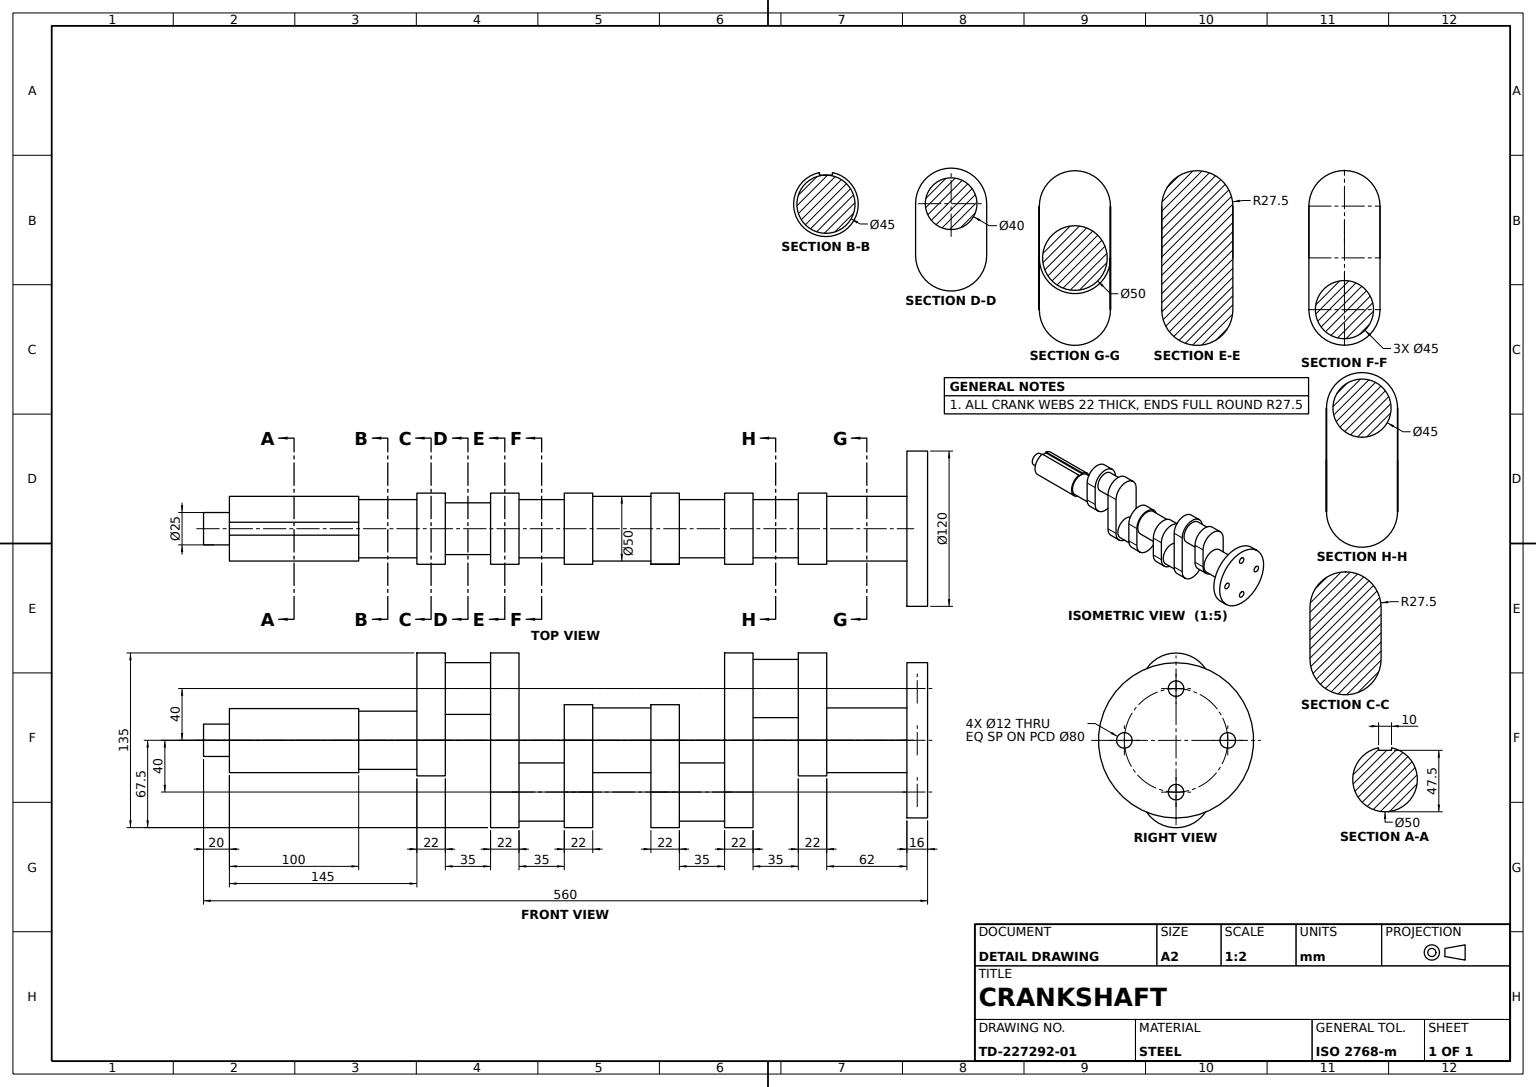
from build123d import *

# Parameters (mm, degrees)
FLANGE_SKETCH_R               = 60
FLANGE_120X16_DEPTH           = 16
FRONT_SHAFT_SKETCH_R          = 25
FRONT_SHAFT_50X62_DEPTH       = 62
CRANK_WEB_1_DEPTH             = 22
CRANKPIN_1_SKETCH_R           = 22.5
CRANKPIN_1_45_DEPTH           = 35
CRANK_WEB_2_DEPTH             = 22
CRANKPIN_2_SKETCH_R           = 22.5
CRANKPIN_2_45_DEPTH           = 35
CRANK_WEB_3_DEPTH             = 22
CENTRE_MAIN_JOURNAL_SKETCH_R  = 25
CENTRE_MAIN_JOURNAL_50_DEPTH  = 45
CRANK_WEB_4_DEPTH             = 22
CRANKPIN_3_SKETCH_R           = 22.5
CRANKPIN_3_45_DEPTH           = 35
CRANK_WEB_5_DEPTH             = 22
CRANKPIN_4_SKETCH_R           = 20
CRANKPIN_4_40_DEPTH           = 35
CRANK_WEB_6_DEPTH             = 22
REAR_SHAFT_SKETCH_R           = 22.5
REAR_SHAFT_45X145_DEPTH       = 145
REAR_START                    = -100
REAR_SHAFT_STEP_SKETCH_R      = 25
REAR_SHAFT_STEP_50X100_DEPTH  = 100
REAR_SHAFT_PROFILE_CUT_DEPTH  = 100
END_STUB_SKETCH_R             = 12.5
END_STUB_25X20_DEPTH          = 20
FLANGE_BOLT_HOLES_SKETCH_R    = 6
FLANGE_BOLT_HOLES_4X_12_DEPTH = 20


with BuildPart() as part:
    # Flange Sketch → Flange Ø120x16 (new body)
    with BuildSketch(Plane.XY):
        Circle(FLANGE_SKETCH_R)
    extrude(amount=FLANGE_120X16_DEPTH)

    # Front Shaft Sketch → Front Shaft Ø50x62 (add)
    with BuildSketch(Plane.XY.offset(16)):
        Circle(FRONT_SHAFT_SKETCH_R)
    extrude(amount=FRONT_SHAFT_50X62_DEPTH)

    # Crank Web 1 Sketch → Crank Web 1 (add)
    with BuildSketch(Plane.XY.offset(78)):
        with BuildLine():
            Line((0, -27.5), (-40, -27.5))
            ThreePointArc((-40, -27.5), (-67.5, 0), (-40, 27.5))
            Line((-40, 27.5), (0, 27.5))
            ThreePointArc((0, 27.5), (27.5, 0), (0, -27.5))
        make_face()
    extrude(amount=CRANK_WEB_1_DEPTH)

    # Crankpin 1 Sketch → Crankpin 1 Ø45 (add)
    with BuildSketch(Plane.XY.offset(100)):
        with Locations((-40, 0)):
            Circle(CRANKPIN_1_SKETCH_R)
    extrude(amount=CRANKPIN_1_45_DEPTH)

    # Crank Web 2 Sketch → Crank Web 2 (add)
    with BuildSketch(Plane.XY.offset(135)):
        with BuildLine():
            Line((-40, 27.5), (40, 27.5))
            ThreePointArc((40, 27.5), (67.5, 0), (40, -27.5))
            Line((40, -27.5), (-40, -27.5))
            ThreePointArc((-40, -27.5), (-67.5, 0), (-40, 27.5))
        make_face()
    extrude(amount=CRANK_WEB_2_DEPTH)

    # Crankpin 2 Sketch → Crankpin 2 Ø45 (add)
    with BuildSketch(Plane.XY.offset(157)):
        with Locations((40, 0)):
            Circle(CRANKPIN_2_SKETCH_R)
    extrude(amount=CRANKPIN_2_45_DEPTH)

    # Crank Web 3 Sketch → Crank Web 3 (add)
    with BuildSketch(Plane.XY.offset(192)):
        with BuildLine():
            Line((40, -27.5), (0, -27.5))
            ThreePointArc((0, -27.5), (-27.5, 0), (0, 27.5))
            Line((0, 27.5), (40, 27.5))
            ThreePointArc((40, 27.5), (67.5, 0), (40, -27.5))
        make_face()
    extrude(amount=CRANK_WEB_3_DEPTH)

    # Centre Main Journal Sketch → Centre Main Journal Ø50 (add)
    with BuildSketch(Plane.XY.offset(214)):
        Circle(CENTRE_MAIN_JOURNAL_SKETCH_R)
    extrude(amount=CENTRE_MAIN_JOURNAL_50_DEPTH)

    # Crank Web 4 Sketch → Crank Web 4 (add)
    with BuildSketch(Plane.XY.offset(259)):
        with BuildLine():
            Line((0, 27.5), (40, 27.5))
            ThreePointArc((40, 27.5), (67.5, 0), (40, -27.5))
            Line((40, -27.5), (0, -27.5))
            ThreePointArc((0, -27.5), (-27.5, 0), (0, 27.5))
        make_face()
    extrude(amount=CRANK_WEB_4_DEPTH)

    # Crankpin 3 Sketch → Crankpin 3 Ø45 (add)
    with BuildSketch(Plane.XY.offset(281)):
        with Locations((40, 0)):
            Circle(CRANKPIN_3_SKETCH_R)
    extrude(amount=CRANKPIN_3_45_DEPTH)

    # Crank Web 5 Sketch → Crank Web 5 (add)
    with BuildSketch(Plane.XY.offset(316)):
        with BuildLine():
            Line((40, -27.5), (-40, -27.5))
            ThreePointArc((-40, -27.5), (-67.5, 0), (-40, 27.5))
            Line((-40, 27.5), (40, 27.5))
            ThreePointArc((40, 27.5), (67.5, 0), (40, -27.5))
        make_face()
    extrude(amount=CRANK_WEB_5_DEPTH)

    # Crankpin 4 Sketch → Crankpin 4 Ø40 (add)
    with BuildSketch(Plane.XY.offset(338)):
        with Locations((-40, 0)):
            Circle(CRANKPIN_4_SKETCH_R)
    extrude(amount=CRANKPIN_4_40_DEPTH)

    # Crank Web 6 Sketch → Crank Web 6 (add)
    with BuildSketch(Plane.XY.offset(373)):
        with BuildLine():
            Line((-40, 27.5), (0, 27.5))
            ThreePointArc((0, 27.5), (27.5, 0), (0, -27.5))
            Line((0, -27.5), (-40, -27.5))
            ThreePointArc((-40, -27.5), (-67.5, 0), (-40, 27.5))
        make_face()
    extrude(amount=CRANK_WEB_6_DEPTH)

    # Rear Shaft Sketch → Rear Shaft Ø45x145 (add)
    with BuildSketch(Plane.XY.offset(395)):
        Circle(REAR_SHAFT_SKETCH_R)
    extrude(amount=REAR_SHAFT_45X145_DEPTH)

    # Rear Shaft Step Sketch → Rear Shaft Step Ø50x100 (add)
    with BuildSketch(Plane.XY.offset(540).offset(REAR_START)):
        Circle(REAR_SHAFT_STEP_SKETCH_R)
    extrude(amount=REAR_SHAFT_STEP_50X100_DEPTH)

    # Rear Shaft Cut Sketch → Rear Shaft Profile Cut (cut)
    with BuildSketch(Plane.XY.offset(540).offset(REAR_START)):
        with BuildLine():
            Line((-24.494897428, -5), (-22.5, -5))
            Line((-22.5, -5), (-22.5, 5))
            Line((-22.5, 5), (-24.494897428, 5))
            ThreePointArc((-24.494897428, 5), (-25, 0), (-24.494897428, -5))
        make_face()
    extrude(amount=REAR_SHAFT_PROFILE_CUT_DEPTH, mode=Mode.SUBTRACT)

    # End Stub Sketch → End Stub Ø25x20 (add)
    with BuildSketch(Plane.XY.offset(540)):
        Circle(END_STUB_SKETCH_R)
    extrude(amount=END_STUB_25X20_DEPTH)

    # Flange Bolt Holes Sketch → Flange Bolt Holes 4xØ12 (cut)
    with BuildSketch(Plane.XY.offset(16)):
        with Locations((0, 40)):
            Circle(FLANGE_BOLT_HOLES_SKETCH_R)
        with Locations((0, -40)):
            Circle(FLANGE_BOLT_HOLES_SKETCH_R)
        with Locations((-40, 0)):
            Circle(FLANGE_BOLT_HOLES_SKETCH_R)
        with Locations((40, 0)):
            Circle(FLANGE_BOLT_HOLES_SKETCH_R)
    extrude(amount=-FLANGE_BOLT_HOLES_4X_12_DEPTH, mode=Mode.SUBTRACT)


solid = part.part
